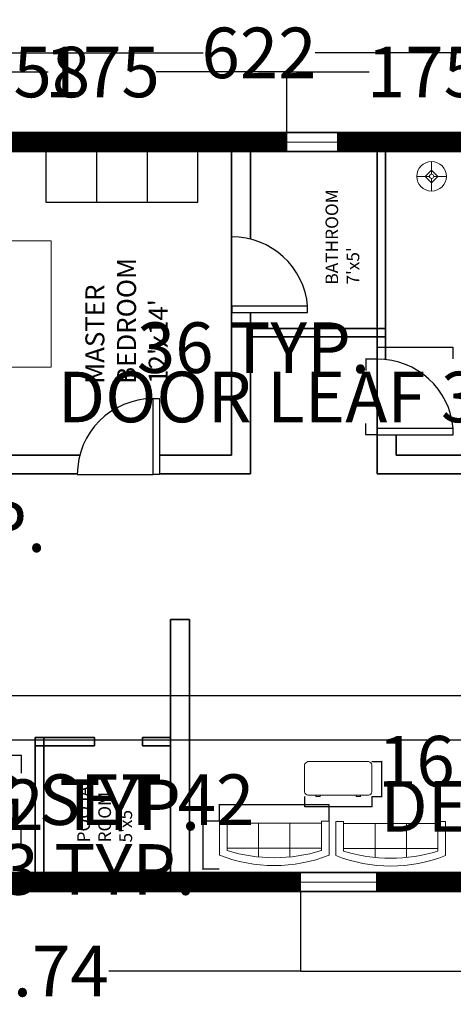
# Model space of a CAD drawing. Units: inches. Extents: x -1226 to 4538, y -998 to 1029.
# Tile 3 of 5: x -864 to -658, y -998 to -531. Entities that reach past the tile are written whole.
import ezdxf

# ---------------------------------------------------------------- set-up
doc = ezdxf.new("R2010")
doc.units = ezdxf.units.IN
doc.header["$MEASUREMENT"] = 0
for name, color, linetype, lineweight in [('A-ANNO-DIMS', 2, 'Continuous', 18), ('A-AREA-IDEN', 7, 'Continuous', 18), ('A-DOOR', 4, 'Continuous', 25), ('A-FLOR-CASE', 8, 'Continuous', 25), ('A-FURN', 8, 'Continuous', 18), ('A-GLAZ', 3, 'Continuous', 18), ('A-WALL', 7, 'Continuous', 35), ('A-WALL-PATT', 1, 'Continuous', 13)]:
    doc.layers.add(name, color=color, linetype=linetype, lineweight=lineweight)
doc.styles.get("Standard").update_dxf_attribs({"font": 'arial.ttf'})
doc.dimstyles.get("Standard").update_dxf_attribs({"dimtxt": 24, "dimasz": 0.18, "dimexe": 0.18, "dimexo": 0.0625, "dimgap": 0.09, "dimtad": 0, "dimtih": 1, "dimtoh": 1, "dimdec": 0, "dimzin": 0, "dimdsep": 46, "dimlunit": 4, "dimtxsty": 'Standard', "dimcen": 0.09, "dimadec": 0, "dimazin": 0, "dimtfac": 1, "dimtdec": 0, "dimtofl": 0, "dimtmove": 0, "dimatfit": 3, "dimfxl": 1, "dimtolj": 1, "dimtzin": 0, "dimarcsym": 0})

# ---------------------------------------------------------------- blocks, each defined once
blk = doc.blocks.new('Desk - 30 x 60 in.')
for p, q in [((-26.999995, 0), (26.999995, 0)), ((-29.999995, -27), (-29.999995, -3)), ((29.999995, -3), (29.999995, -27)), ((26.999995, -30), (-26.999995, -30)), ((-20.000005, -30), (-20.000005, -31)), ((-20.000005, -31), (-16.000005, -31)), ((-16.000005, -31), (-16.000005, -30)), ((15.999995, -31), (15.999995, -30)), ((19.999995, -31), (15.999995, -31)), ((19.999995, -30), (19.999995, -31))]:
    blk.add_line(p, q)
for centre, start, end in [((-26.499995, -3.5), 98.1301, 171.8699), ((26.499995, -3.5), 8.130102, 81.8699), ((-26.499995, -26.5), 188.1301, 261.8699), ((26.499995, -26.5), 278.1301, 351.8699)]:
    blk.add_arc(centre, 3.535534, start, end)
blk = doc.blocks.new('Sofa - Roundback 7 ft.')
for p, q in [((-12.00002, -32.4421), (-12.00003, -6.5971)), ((11.99997, -32.4421), (11.99998, -6.5971)), ((-36.000027, -34), (-36.000027, -11.4696)), ((-35.999844, -13.3819), (35.9998, -13.3819)), ((35.99998, -34), (35.99998, -11.4696)), ((-36.000027, -32.4421), (35.99998, -32.4421))]:
    blk.add_line(p, q)
for points in [[(-36.000027, -34), (-42.000027, -34), (-42.000027, -8)], [(41.99998, -8), (41.99998, -34), (35.99998, -34)]]:
    blk.add_lwpolyline(points)
for centre, radius, start, end in [((0, -114.25), 114.25, 68.43141, 111.5686), ((-0.00001, -127.1968), 121.1968, 72.72033, 107.2797)]:
    blk.add_arc(centre, radius, start, end)
blk = doc.blocks.new('Bed - Queen')
for p, q in [((0, -80.00003), (0, 0)), ((0, 0), (59.99999, 0)), ((59.99999, 0), (59.99999, -80.00003)), ((7.99999, -1.2), (28.79998, -1.2)), ((7.99999, -14.4), (7.99999, -1.2)), ((28.79998, -1.2), (28.79998, -14.4)), ((31.19999, -1.2), (51.99999, -1.2)), ((31.19999, -14.4), (31.19999, -1.2)), ((51.99999, -1.2), (51.99999, -16.4)), ((0, -14.4), (44.8, -14.4)), ((44.8, -16.8), (0, -16.8)), ((59.99999, -29.6), (44.8, -14.4)), ((44.8, -14.4), (44.8, -29.6)), ((51.99999, -16.4), (46.79936, -16.4)), ((44.8, -29.6), (59.99999, -29.6)), ((59.99999, -80.00003), (0, -80.00003))]:
    blk.add_line(p, q)
blk = doc.blocks.new('Lamp - Table')
for p, q in [((0, 7), (0, 1)), ((-1, 0), (-7, 0)), ((0, 3), (-3, 0)), ((-3, 0), (0, -3)), ((3, 0), (0, 3)), ((0, -3), (3, 0)), ((1, 0), (7, 0)), ((0, -1), (0, -7))]:
    blk.add_line(p, q)
for radius in [7, 1]:
    blk.add_circle((0, 0), radius)
blk = doc.blocks.new('DOOR-SWING-36')
for p, q in [((36, 36), (0, 36)), ((0, 36), (0, 33)), ((0, 33), (36, 33)), ((36, 33), (36, 36))]:
    blk.add_line(p, q)
blk.add_arc((36, 36.14), 36.14, 184.9791, 270)
blk = doc.blocks.new('WIN-36')
for p, q in [((0, 36), (9, 36)), ((4.5, 0), (4.5, 36)), ((0, 0), (9, 0))]:
    blk.add_line(p, q)
blk = doc.blocks.new('WIN-24')
for p, q in [((0, 24), (9, 24)), ((4.5, 0), (4.5, 24)), ((0, 0), (9, 0))]:
    blk.add_line(p, q)
blk = doc.blocks.new('WARDROBE-72X24')
for p, q in [((72, 24), (0, 24)), ((0, 24), (0, 0)), ((24, 24), (24, 0)), ((48, 24), (48, 0)), ((72, 0), (72, 24)), ((0, 0), (72, 0))]:
    blk.add_line(p, q)
blk = doc.blocks.new('*D26')
at = {"layer": 'A-ANNO-DIMS', "color": 0, "lineweight": -2, "transparency": 16777216}
for p, q in [((-694.2, -692), (-699.72, -692)), ((-699.54, -692.18), (-699.54, -697.48)), ((-699.54, -727.82), (-699.54, -722.51)), ((-694.2, -728), (-699.72, -728))]:
    blk.add_line(p, q, dxfattribs=at)
at = {"layer": 'A-ANNO-DIMS', "color": 0, "transparency": 16777216}
for points in [[(-699.57, -692.18), (-699.51, -692.18), (-699.54, -692)], [(-699.57, -727.82), (-699.51, -727.82), (-699.54, -728)]]:
    blk.add_solid(points, dxfattribs=at)
at = {"layer": 'Defpoints', "color": 0, "transparency": 16777216}
for p in [(-694.14, -692), (-699.54, -728), (-694.14, -728)]:
    blk.add_point(p, dxfattribs=at)
at = {"layer": 'A-ANNO-DIMS', "color": 0, "transparency": 16777216, "insert": (-699.54, -710), "char_height": 24, "attachment_point": 5}
blk.add_mtext('\\A1;DOOR LEAF 36 TYP.', dxfattribs=at)
blk = doc.blocks.new('*D27')
at = {"layer": 'A-ANNO-DIMS', "color": 0, "lineweight": -2, "transparency": 16777216}
for p, q in [((-694.14, -691.93), (-694.14, -686.42)), ((-658.14, -691.93), (-658.14, -686.42)), ((-694.14, -686.6), (-694.32, -686.6)), ((-658.32, -686.6), (-693.96, -686.6))]:
    blk.add_line(p, q, dxfattribs=at)
at = {"layer": 'A-ANNO-DIMS', "color": 0, "transparency": 16777216}
for points in [[(-693.96, -686.57), (-693.96, -686.63), (-694.14, -686.6)], [(-658.32, -686.57), (-658.32, -686.63), (-658.14, -686.6)]]:
    blk.add_solid(points, dxfattribs=at)
at = {"layer": 'Defpoints', "color": 0, "transparency": 16777216}
for p in [(-694.14, -686.6), (-694.14, -692), (-658.14, -692)]:
    blk.add_point(p, dxfattribs=at)
at = {"layer": 'A-ANNO-DIMS', "color": 0, "transparency": 16777216, "insert": (-752.81, -686.6), "char_height": 24, "attachment_point": 5}
blk.add_mtext('\\A1;36 TYP.', dxfattribs=at)
blk = doc.blocks.new('*D28')
at = {"layer": 'A-ANNO-DIMS', "color": 0, "lineweight": -2, "transparency": 16777216}
for p, q in [((-1080.03, -767.33), (-1080.03, -771.62)), ((-1052.19, -767.33), (-1052.19, -771.62)), ((-1079.85, -771.44), (-1052.37, -771.44)), ((-1052.19, -771.44), (-1052.01, -771.44))]:
    blk.add_line(p, q, dxfattribs=at)
at = {"layer": 'A-ANNO-DIMS', "color": 0, "transparency": 16777216}
for points in [[(-1079.85, -771.41), (-1079.85, -771.47), (-1080.03, -771.44)], [(-1052.37, -771.41), (-1052.37, -771.47), (-1052.19, -771.44)]]:
    blk.add_solid(points, dxfattribs=at)
at = {"layer": 'Defpoints', "color": 0, "transparency": 16777216}
for p in [(-1080.03, -767.26), (-1052.19, -767.26), (-1052.19, -771.44)]:
    blk.add_point(p, dxfattribs=at)
at = {"layer": 'A-ANNO-DIMS', "color": 0, "transparency": 16777216, "insert": (-947.45, -771.44), "char_height": 24, "attachment_point": 5}
blk.add_mtext('\\A1;LEAF 28 TYP.', dxfattribs=at)
blk = doc.blocks.new('*D34')
at = {"layer": 'A-ANNO-DIMS', "color": 0, "lineweight": -2, "transparency": 16777216}
for p, q in [((-768.95, -903.42), (-769.13, -903.42)), ((-768.95, -911.16), (-768.95, -903.24)), ((-717.1, -903.42), (-768.77, -903.42)), ((-716.92, -911.16), (-716.92, -903.24))]:
    blk.add_line(p, q, dxfattribs=at)
at = {"layer": 'A-ANNO-DIMS', "color": 0, "transparency": 16777216}
for points in [[(-768.77, -903.39), (-768.77, -903.45), (-768.95, -903.42)], [(-717.1, -903.39), (-717.1, -903.45), (-716.92, -903.42)]]:
    blk.add_solid(points, dxfattribs=at)
at = {"layer": 'Defpoints', "color": 0, "transparency": 16777216}
for p in [(-768.95, -903.42), (-768.95, -911.22), (-716.92, -911.22)]:
    blk.add_point(p, dxfattribs=at)
at = {"layer": 'A-ANNO-DIMS', "color": 0, "transparency": 16777216, "insert": (-877.88, -903.42), "char_height": 24, "attachment_point": 5}
blk.add_mtext('\\A1;SOFA 52 TYP.', dxfattribs=at)
blk = doc.blocks.new('*D35')
at = {"layer": 'A-ANNO-DIMS', "color": 0, "lineweight": -2, "transparency": 16777216}
for p, q in [((-769.01, -911.22), (-776.94, -911.22)), ((-776.76, -911.4), (-776.76, -933.75)), ((-769.01, -933.93), (-776.94, -933.93)), ((-776.76, -933.93), (-776.76, -934.11)), ((-776.76, -934.11), (-776.94, -934.11))]:
    blk.add_line(p, q, dxfattribs=at)
at = {"layer": 'A-ANNO-DIMS', "color": 0, "transparency": 16777216}
for points in [[(-776.79, -911.4), (-776.73, -911.4), (-776.76, -911.22)], [(-776.79, -933.75), (-776.73, -933.75), (-776.76, -933.93)]]:
    blk.add_solid(points, dxfattribs=at)
at = {"layer": 'Defpoints', "color": 0, "transparency": 16777216}
for p in [(-768.95, -911.22), (-776.76, -933.93), (-768.95, -933.93)]:
    blk.add_point(p, dxfattribs=at)
at = {"layer": 'A-ANNO-DIMS', "color": 0, "transparency": 16777216, "insert": (-835.64, -934.11), "char_height": 24, "attachment_point": 5}
blk.add_mtext('\\A1;23 TYP.', dxfattribs=at)
blk = doc.blocks.new('*D44')
at = {"layer": 'A-ANNO-DIMS', "color": 0, "lineweight": -2, "transparency": 16777216}
for p, q in [((-728.59, -899.5), (-728.59, -904.39)), ((-696.71, -899.5), (-696.71, -904.39)), ((-728.41, -904.21), (-696.89, -904.21)), ((-696.71, -904.21), (-696.53, -904.21))]:
    blk.add_line(p, q, dxfattribs=at)
at = {"layer": 'A-ANNO-DIMS', "color": 0, "transparency": 16777216}
for points in [[(-728.41, -904.18), (-728.41, -904.24), (-728.59, -904.21)], [(-696.89, -904.18), (-696.89, -904.24), (-696.71, -904.21)]]:
    blk.add_solid(points, dxfattribs=at)
at = {"layer": 'Defpoints', "color": 0, "transparency": 16777216}
for p in [(-728.59, -899.43), (-696.71, -899.43), (-696.71, -904.21)]:
    blk.add_point(p, dxfattribs=at)
at = {"layer": 'A-ANNO-DIMS', "color": 0, "transparency": 16777216, "insert": (-629.67, -904.21), "char_height": 24, "attachment_point": 5}
blk.add_mtext('\\A1;DESK 32', dxfattribs=at)
blk = doc.blocks.new('*D45')
at = {"layer": 'A-ANNO-DIMS', "color": 0, "lineweight": -2, "transparency": 16777216}
for p, q in [((-696.65, -882.96), (-691.75, -882.96)), ((-691.93, -882.96), (-691.93, -882.78)), ((-691.93, -882.78), (-691.75, -882.78)), ((-691.93, -899.25), (-691.93, -883.14)), ((-696.65, -899.43), (-691.75, -899.43))]:
    blk.add_line(p, q, dxfattribs=at)
at = {"layer": 'A-ANNO-DIMS', "color": 0, "transparency": 16777216}
for points in [[(-691.96, -883.14), (-691.9, -883.14), (-691.93, -882.96)], [(-691.96, -899.25), (-691.9, -899.25), (-691.93, -899.43)]]:
    blk.add_solid(points, dxfattribs=at)
at = {"layer": 'Defpoints', "color": 0, "transparency": 16777216}
for p in [(-696.71, -882.96), (-691.93, -882.96), (-696.71, -899.43)]:
    blk.add_point(p, dxfattribs=at)
at = {"layer": 'A-ANNO-DIMS', "color": 0, "transparency": 16777216, "insert": (-675.61, -882.78), "char_height": 24, "attachment_point": 5}
blk.add_mtext('\\A1;16', dxfattribs=at)
blk = doc.blocks.new('*D46')
at = {"layer": 'A-ANNO-DIMS', "color": 0, "lineweight": -2, "transparency": 16777216}
for p, q in [((-869.17, -879.93), (-862.73, -879.93)), ((-862.91, -880.11), (-862.91, -888.51)), ((-862.91, -921.91), (-862.91, -913.51)), ((-869.17, -922.09), (-862.73, -922.09))]:
    blk.add_line(p, q, dxfattribs=at)
at = {"layer": 'A-ANNO-DIMS', "color": 0, "transparency": 16777216}
for points in [[(-862.94, -880.11), (-862.88, -880.11), (-862.91, -879.93)], [(-862.94, -921.91), (-862.88, -921.91), (-862.91, -922.09)]]:
    blk.add_solid(points, dxfattribs=at)
at = {"layer": 'Defpoints', "color": 0, "transparency": 16777216}
for p in [(-869.23, -879.93), (-862.91, -879.93), (-869.23, -922.09)]:
    blk.add_point(p, dxfattribs=at)
at = {"layer": 'A-ANNO-DIMS', "color": 0, "transparency": 16777216, "insert": (-862.91, -901.01), "char_height": 24, "attachment_point": 5}
blk.add_mtext('\\A1;DINING SET 42', dxfattribs=at)
blk = doc.blocks.new('*D48')
at = {"layer": 'A-ANNO-DIMS', "color": 0, "lineweight": -2, "transparency": 16777216}
for p, q in [((-1061.17, -584.46), (-1061.17, -546.6)), ((-1060.99, -546.78), (-776.71, -546.78)), ((-439.35, -546.78), (-723.62, -546.78)), ((-439.17, -584.46), (-439.17, -546.6))]:
    blk.add_line(p, q, dxfattribs=at)
at = {"layer": 'A-ANNO-DIMS', "color": 0, "transparency": 16777216}
for points in [[(-1060.99, -546.75), (-1060.99, -546.81), (-1061.17, -546.78)], [(-439.35, -546.75), (-439.35, -546.81), (-439.17, -546.78)]]:
    blk.add_solid(points, dxfattribs=at)
at = {"layer": 'Defpoints', "color": 0, "transparency": 16777216}
for p in [(-439.17, -546.78), (-1061.17, -584.53), (-439.17, -584.53)]:
    blk.add_point(p, dxfattribs=at)
at = {"layer": 'A-ANNO-DIMS', "color": 0, "transparency": 16777216, "insert": (-750.17, -546.78), "char_height": 24, "attachment_point": 5}
blk.add_mtext('\\A1;622', dxfattribs=at)
blk = doc.blocks.new('*D52')
at = {"layer": 'A-ANNO-DIMS', "color": 0, "lineweight": -2, "transparency": 16777216}
for p, q in [((-974.51, -593.51), (-974.49, -555.64)), ((-911.93, -593.53), (-911.92, -555.66)), ((-974.31, -555.82), (-912.1, -555.84)), ((-911.92, -555.84), (-911.74, -555.84))]:
    blk.add_line(p, q, dxfattribs=at)
at = {"layer": 'A-ANNO-DIMS', "color": 0, "transparency": 16777216}
for points in [[(-974.31, -555.79), (-974.31, -555.85), (-974.49, -555.82)], [(-912.1, -555.81), (-912.1, -555.87), (-911.92, -555.84)]]:
    blk.add_solid(points, dxfattribs=at)
at = {"layer": 'Defpoints', "color": 0, "transparency": 16777216}
for p in [(-911.92, -555.84), (-974.51, -593.57), (-911.93, -593.59)]:
    blk.add_point(p, dxfattribs=at)
at = {"layer": 'A-ANNO-DIMS', "color": 0, "transparency": 16777216, "insert": (-871.06, -555.84), "char_height": 24, "attachment_point": 5}
blk.add_mtext('\\A1;62.58', dxfattribs=at)
blk = doc.blocks.new('*D53')
at = {"layer": 'A-ANNO-DIMS', "color": 0, "lineweight": -2, "transparency": 16777216}
for p, q in [((-911.93, -593.53), (-911.94, -555.66)), ((-736.92, -593.48), (-736.93, -555.62)), ((-911.76, -555.84), (-850, -555.82)), ((-737.11, -555.8), (-798.87, -555.81))]:
    blk.add_line(p, q, dxfattribs=at)
at = {"layer": 'A-ANNO-DIMS', "color": 0, "transparency": 16777216}
for points in [[(-737.11, -555.77), (-737.11, -555.83), (-736.93, -555.8)], [(-911.76, -555.81), (-911.76, -555.87), (-911.94, -555.84)]]:
    blk.add_solid(points, dxfattribs=at)
at = {"layer": 'Defpoints', "color": 0, "transparency": 16777216}
for p in [(-736.93, -555.8), (-911.93, -593.59), (-736.92, -593.55)]:
    blk.add_point(p, dxfattribs=at)
at = {"layer": 'A-ANNO-DIMS', "color": 0, "transparency": 16777216, "insert": (-824.43, -555.82), "char_height": 24, "attachment_point": 5}
blk.add_mtext('\\A1;175', dxfattribs=at)
blk = doc.blocks.new('*D54')
at = {"layer": 'A-ANNO-DIMS', "color": 0, "lineweight": -2, "transparency": 16777216}
for p, q in [((-736.92, -593.48), (-736.92, -555.62)), ((-736.74, -555.8), (-697.91, -555.79)), ((-561.35, -555.78), (-600.18, -555.78)), ((-561.17, -593.46), (-561.17, -555.6))]:
    blk.add_line(p, q, dxfattribs=at)
at = {"layer": 'A-ANNO-DIMS', "color": 0, "transparency": 16777216}
for points in [[(-736.74, -555.77), (-736.74, -555.83), (-736.92, -555.8)], [(-561.35, -555.75), (-561.35, -555.81), (-561.17, -555.78)]]:
    blk.add_solid(points, dxfattribs=at)
at = {"layer": 'Defpoints', "color": 0, "transparency": 16777216}
for p in [(-561.17, -555.78), (-736.92, -593.55), (-561.17, -593.53)]:
    blk.add_point(p, dxfattribs=at)
at = {"layer": 'A-ANNO-DIMS', "color": 0, "transparency": 16777216, "insert": (-649.05, -555.79), "char_height": 24, "attachment_point": 5}
blk.add_mtext('\\A1;175.75', dxfattribs=at)
blk = doc.blocks.new('*D57')
at = {"layer": 'A-ANNO-DIMS', "color": 0, "lineweight": -2, "transparency": 16777216}
for p, q in [((-1012.21, -944.64), (-1012.21, -982.51)), ((-730.47, -944.64), (-730.47, -982.51)), ((-1012.03, -982.33), (-921.41, -982.33)), ((-730.65, -982.33), (-821.28, -982.33))]:
    blk.add_line(p, q, dxfattribs=at)
at = {"layer": 'A-ANNO-DIMS', "color": 0, "transparency": 16777216}
for points in [[(-1012.03, -982.3), (-1012.03, -982.36), (-1012.21, -982.33)], [(-730.65, -982.3), (-730.65, -982.36), (-730.47, -982.33)]]:
    blk.add_solid(points, dxfattribs=at)
at = {"layer": 'Defpoints', "color": 0, "transparency": 16777216}
for p in [(-1012.21, -944.57), (-730.47, -944.58), (-730.47, -982.33)]:
    blk.add_point(p, dxfattribs=at)
at = {"layer": 'A-ANNO-DIMS', "color": 0, "transparency": 16777216, "insert": (-871.34, -982.33), "char_height": 24, "attachment_point": 5}
blk.add_mtext('\\A1;281.74', dxfattribs=at)
blk = doc.blocks.new('*D58')
at = {"layer": 'A-ANNO-DIMS', "color": 0, "lineweight": -2, "transparency": 16777216}
for p, q in [((-730.47, -944.64), (-730.47, -982.51)), ((-651.08, -944.55), (-651.08, -982.51)), ((-730.29, -982.33), (-651.26, -982.33)), ((-651.08, -982.33), (-650.9, -982.33))]:
    blk.add_line(p, q, dxfattribs=at)
at = {"layer": 'A-ANNO-DIMS', "color": 0, "transparency": 16777216}
for points in [[(-730.29, -982.3), (-730.29, -982.36), (-730.47, -982.33)], [(-651.26, -982.3), (-651.26, -982.36), (-651.08, -982.33)]]:
    blk.add_solid(points, dxfattribs=at)
at = {"layer": 'Defpoints', "color": 0, "transparency": 16777216}
for p in [(-730.47, -944.58), (-651.08, -944.48), (-651.08, -982.33)]:
    blk.add_point(p, dxfattribs=at)
at = {"layer": 'A-ANNO-DIMS', "color": 0, "transparency": 16777216, "insert": (-610.39, -982.33), "char_height": 24, "attachment_point": 5}
blk.add_mtext('\\A1;79.39', dxfattribs=at)
blk = doc.blocks.new('*D78')
at = {"layer": 'A-ANNO-DIMS', "color": 0, "lineweight": -2, "transparency": 16777216}
for p, q in [((-1028.09, -851.56), (-401.24, -851.56)), ((-401.42, -851.74), (-401.42, -872.38)), ((-1028.09, -872.56), (-401.24, -872.56)), ((-401.42, -872.74), (-401.6, -872.74)), ((-401.42, -872.56), (-401.42, -872.74))]:
    blk.add_line(p, q, dxfattribs=at)
at = {"layer": 'A-ANNO-DIMS', "color": 0, "transparency": 16777216}
for points in [[(-401.45, -851.74), (-401.39, -851.74), (-401.42, -851.56)], [(-401.45, -872.38), (-401.39, -872.38), (-401.42, -872.56)]]:
    blk.add_solid(points, dxfattribs=at)
at = {"layer": 'Defpoints', "color": 0, "transparency": 16777216}
for p in [(-1028.16, -851.56), (-1028.16, -872.56), (-401.42, -872.56)]:
    blk.add_point(p, dxfattribs=at)
at = {"layer": 'A-ANNO-DIMS', "color": 0, "transparency": 16777216, "insert": (-416.76, -872.74), "char_height": 24, "attachment_point": 5}
blk.add_mtext('\\A1;21', dxfattribs=at)

msp = doc.modelspace()

# ---------------------------------------------------------------- hatches: boundary and pattern name
at = {"layer": 'A-WALL-PATT'}
h = msp.add_hatch(dxfattribs=at)
h.set_pattern_fill('ANSI31', color=256, angle=90)
h.set_pattern_definition([(135, (-1048.80633, 527.86775), (-0.088388348, -0.088388348), [])])
h.paths.add_polyline_path([(-1052.1662, -935.5274), (-1052.1662, -878.4295), (-1061.1662, -878.4295), (-1061.1662, -944.5274), (-1012.2132, -944.5274), (-1012.2132, -935.5274)])
h.paths.add_polyline_path([(-976.2132, -935.5274), (-976.2132, -944.5274), (-730.4734, -944.5274), (-730.4734, -935.5274)])
h.paths.add_polyline_path([(-694.4734, -935.5274), (-694.4734, -944.5274), (-651.0832, -944.5274), (-651.0832, -935.5274)])
h.paths.add_polyline_path([(-615.0832, -935.5274), (-615.0832, -944.5274), (-561.1662, -944.5274), (-561.1662, -935.5274)])
h.paths.add_polyline_path([(-712.9165, -584.5274), (-712.9165, -593.5274), (-657.3138, -593.5274), (-657.3138, -593.4838), (-597.3139, -593.4838), (-448.1662, -593.5274), (-448.1662, -713.5274), (-448.1662, -779.5274), (-439.1662, -779.5274), (-439.1662, -584.5274)])
h.paths.add_polyline_path([(-875.9292, -584.5274), (-875.9292, -593.5274), (-736.9165, -593.5274), (-736.9165, -584.5274)])
h.paths.add_polyline_path([(-950.5052, -584.5274), (-950.5052, -593.5274), (-911.9292, -593.5274), (-911.9292, -584.5274)])
h.paths.add_polyline_path([(-1011.0429, -584.5274), (-1011.0429, -593.5274), (-974.5052, -593.5274), (-974.5052, -584.5274)])
h.paths.add_polyline_path([(-1061.1662, -584.5274), (-1061.1662, -693.4459), (-1052.1662, -693.4459), (-1052.1662, -593.5274), (-1035.0429, -593.5274), (-1035.0429, -584.5274)])
h.paths.add_polyline_path([(-1061.1662, -795.2404), (-1061.1662, -842.4295), (-1052.1662, -842.4295), (-1052.1662, -795.2404)])
h.paths.add_polyline_path([(-1061.1662, -717.4459), (-1061.1662, -739.4249), (-1052.1662, -739.4249), (-1052.1662, -717.4459)])

# ---------------------------------------------------------------- linework, layer by layer
at = {"layer": 'A-DOOR'}
for p, q in [((-800.2652, -746.7644), (-800.2652, -710.7644)), ((-800.2652, -710.7644), (-797.2652, -710.7644)), ((-797.2652, -710.7644), (-797.2652, -746.7644)), ((-836.2652, -746.7644), (-800.2652, -746.7644)), ((-797.2652, -746.7644), (-800.2652, -746.7644))]:
    msp.add_line(p, q, dxfattribs=at)
msp.add_arc((-800.2652, -746.7644), 36, 90, 180, dxfattribs=at)
at = {"layer": 'A-WALL'}
for p, q in [((-1061.1662, -584.5274), (-439.1662, -584.5274)), ((-1052.1662, -593.5274), (-448.1662, -593.5274)), ((-763.1662, -737.5274), (-763.1662, -593.5274)), ((-754.1662, -635.1105), (-754.1662, -593.5274)), ((-694.1662, -746.5274), (-694.1662, -593.5274)), ((-690.1662, -692.2149), (-690.1662, -593.5274)), ((-754.1662, -746.5274), (-754.1662, -669.9829)), ((-754.1662, -677.5274), (-690.1662, -677.5274)), ((-754.1662, -681.5274), (-690.1662, -681.5274)), ((-685.1662, -737.5274), (-685.1662, -727.9957)), ((-931.1662, -737.5274), (-835.06, -737.5274)), ((-797.2652, -737.5274), (-763.1662, -737.5274)), ((-685.1662, -737.5274), (-570.1662, -737.5274)), ((-940.1662, -746.5274), (-836.2644, -746.5274)), ((-797.2652, -746.5274), (-754.1662, -746.5274)), ((-694.1662, -746.5274), (-570.1662, -746.5274)), ((-792.1662, -935.5274), (-792.1662, -815.5274)), ((-792.1662, -815.5274), (-783.1662, -815.5274)), ((-783.1662, -935.5274), (-783.1662, -815.5274)), ((-856.1662, -935.5274), (-856.1662, -871.5274)), ((-856.1662, -871.5274), (-828.1662, -871.5274)), ((-852.1662, -935.5274), (-852.1662, -871.5274)), ((-828.1662, -875.5274), (-828.1662, -871.5274)), ((-805.3868, -875.5274), (-805.3868, -871.5274)), ((-805.3868, -871.5274), (-798.1662, -871.5274)), ((-798.1662, -871.5274), (-792.1662, -871.5274)), ((-856.1662, -875.5274), (-828.1662, -875.5274)), ((-798.1662, -875.5274), (-805.3868, -875.5274)), ((-798.1662, -875.5274), (-792.1662, -875.5274)), ((-1052.1662, -935.5274), (-439.1662, -935.5274)), ((-1061.1662, -944.5274), (-561.1662, -944.5274))]:
    msp.add_line(p, q, dxfattribs=at)

# ---------------------------------------------------------------- block references
at = {"layer": 'A-DOOR', "rotation": 180}
for p in [(-727.1229, -633.9828), (-658.1407, -691.9955)]:
    msp.add_blockref('DOOR-SWING-36', p, dxfattribs=at)
at = {"layer": 'A-FLOR-CASE'}
msp.add_blockref('WARDROBE-72X24', (-851.221, -617.611), dxfattribs=at)
at = {"layer": 'A-FURN', "rotation": 90}
for name, p in [('Lamp - Table', (-668.409, -605.3515)), ('Bed - Queen', (-928.5798, -695.9107))]:
    msp.add_blockref(name, p, dxfattribs=at)
at = {"layer": 'A-FURN', "xscale": 0.5312748563161357, "yscale": 0.5312748563161357, "zscale": 0.5312748563161357}
msp.add_blockref('Desk - 30 x 60 in.', (-712.6514, -882.9631), dxfattribs=at)
at = {"layer": 'A-FURN', "xscale": 0.6193974930679756, "yscale": 0.6193974930679756, "zscale": 0.6193974930679756, "rotation": 180}
for p in [(-742.937, -932.2828), (-687.7668, -932.4759)]:
    msp.add_blockref('Sofa - Roundback 7 ft.', p, dxfattribs=at)
at = {"layer": 'A-GLAZ'}
for name, p, rotation in [('WIN-24', (-736.9166, -584.5459), 269.9999999999979), ('WIN-36', (-730.4729, -935.5814), 270.0000000000005)]:
    msp.add_blockref(name, p, dxfattribs=dict(at, rotation=rotation))

# ---------------------------------------------------------------- texts
at = {"layer": 'A-AREA-IDEN', "attachment_point": 1, "rotation": 90}
for s, width, heights, insert, char_height in [("BATHROOM\\P7'x5'", 19.792618, [19.7709], (-718.6654, -656.6814), 6), ("MASTER\\PBEDROOM\\P12'x14'", 76.603238, [0], (-832.4425, -703.7693), 9), ("POOJA ROOM\\P5'x5'", 36.971038, [0], (-836.3014, -921.3165), 6)]:
    msp.add_mtext_dynamic_manual_height_columns(s, width=width, gutter_width=1, heights=heights, dxfattribs=dict(at, insert=insert, char_height=char_height))

# ---------------------------------------------------------------- dimensions: what is measured, and where the dimension line sits
at = {"layer": 'A-ANNO-DIMS'}
for base, p1, p2, override, picture, middle in [((-439.1662, -546.7774), (-1061.1662, -584.5274), (-439.1662, -584.5274), {"dimdec": 0, "dimlfac": 1, "dimrnd": 0, "dimzin": 0, "dimdsep": 46, "dimlunit": 2}, '*D48', (-750.1662, -546.7774)), ((-730.4734, -982.3314), (-1012.2132, -944.5741), (-730.4734, -944.5814), {"dimdec": 2, "dimlfac": 1, "dimrnd": 0, "dimzin": 0, "dimdsep": 46, "dimlunit": 2}, '*D57', (-871.3433, -982.3314)), ((-651.0832, -982.3314), (-730.4734, -944.5814), (-651.0832, -944.4838), {"dimdec": 2, "dimlfac": 1, "dimrnd": 0, "dimzin": 0, "dimdsep": 46, "dimlunit": 2}, '*D58', (-610.393, -982.3314))]:
    dim = msp.add_linear_dim(base=base, p1=p1, p2=p2, dimstyle='Standard', override=override, dxfattribs=at)
    dim.commit()
    dim.dimension.update_dxf_attribs({"geometry": picture, "text_midpoint": middle})
for base, p1, p2, angle, override, picture, middle in [((-911.9169, -555.8393), (-974.5052, -593.569), (-911.9292, -593.5893), 359.981403, {"dimdec": 2, "dimlfac": 1, "dimrnd": 0, "dimzin": 0, "dimdsep": 46, "dimlunit": 2}, '*D52', (-871.063, -555.8393)), ((-736.9259, -555.7956), (-911.9292, -593.5893), (-736.9165, -593.5456), 0.014311, {"dimdec": 0, "dimlfac": 1, "dimrnd": 0, "dimzin": 0, "dimdsep": 46, "dimlunit": 2}, '*D53', (-824.4323, -555.8174)), ((-561.1701, -555.7774), (-736.9165, -593.5456), (-561.1662, -593.5274), 0.005909, {"dimdec": 2, "dimlfac": 1, "dimrnd": 0, "dimzin": 0, "dimdsep": 46, "dimlunit": 2}, '*D54', (-649.0452, -555.7865)), ((-401.4162, -872.5639), (-1028.1562, -851.5639), (-1028.1562, -872.5639), 90, {"dimdec": 0, "dimlfac": 1, "dimrnd": 0, "dimzin": 0, "dimdsep": 46, "dimlunit": 2}, '*D78', (-416.7639, -872.7439)), ((-691.9317, -882.9631), (-696.7132, -899.4326), (-696.7132, -882.9631), 90, {"dimdec": 0, "dimlfac": 1, "dimrnd": 0, "dimzin": 0, "dimdsep": 46, "dimlunit": 2}, '*D45', (-675.6099, -882.7831))]:
    dim = msp.add_linear_dim(base=base, p1=p1, p2=p2, angle=angle, dimstyle='Standard', override=override, dxfattribs=at)
    dim.commit()
    dim.dimension.update_dxf_attribs({"geometry": picture, "text_midpoint": middle})
for base, p1, p2, angle, text, picture, middle in [((-699.5403, -727.9957), (-694.1403, -691.9957), (-694.1403, -727.9957), 270, 'DOOR LEAF <> TYP.', '*D26', (-699.5403, -709.9957)), ((-694.1403, -686.5957), (-658.1403, -691.9957), (-694.1403, -691.9957), 180, '<> TYP.', '*D27', (-752.8141, -686.5957)), ((-862.9094, -879.9303), (-869.2335, -922.091), (-869.2335, -879.9303), 90, 'DINING SET <>', '*D46', (-862.9094, -901.0106)), ((-768.9517, -903.4189), (-716.9223, -911.2233), (-768.9517, -911.2233), 180, 'SOFA <> TYP.', '*D34', (-877.8765, -903.4189)), ((-776.7561, -933.9346), (-768.9517, -911.2233), (-768.9517, -933.9346), 270, '<> TYP.', '*D35', (-835.6427, -934.1146))]:
    dim = msp.add_linear_dim(base=base, p1=p1, p2=p2, angle=angle, text=text, dimstyle='Standard', override={"dimdec": 0, "dimlfac": 1, "dimrnd": 0, "dimzin": 0, "dimdsep": 46, "dimlunit": 2}, dxfattribs=at)
    dim.commit()
    dim.dimension.update_dxf_attribs({"geometry": picture, "text_midpoint": middle})
for base, p1, p2, text, picture, middle in [((-1052.1878, -771.4403), (-1080.0272, -767.2643), (-1052.1878, -767.2643), 'LEAF <> TYP.', '*D28', (-947.4539, -771.4403)), ((-696.7132, -904.2141), (-728.5897, -899.4326), (-696.7132, -899.4326), 'DESK <>', '*D44', (-629.6656, -904.2141))]:
    dim = msp.add_linear_dim(base=base, p1=p1, p2=p2, text=text, dimstyle='Standard', override={"dimdec": 0, "dimlfac": 1, "dimrnd": 0, "dimzin": 0, "dimdsep": 46, "dimlunit": 2}, dxfattribs=at)
    dim.commit()
    dim.dimension.update_dxf_attribs({"geometry": picture, "text_midpoint": middle})

doc.saveas('drawing.dxf')
